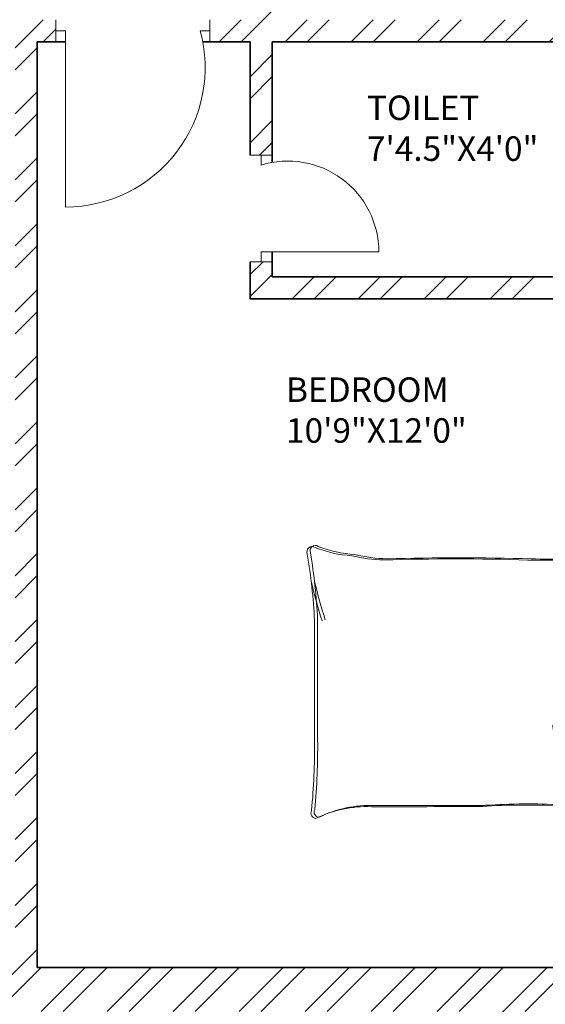
# Model space of a CAD drawing. Units: inches. Extents: x 2120 to 4013, y 1390 to 3019.
# Tile 42 of 59: x 2861 to 2968, y 1964 to 2165. Entities that reach past the tile are written whole.
import ezdxf

# ---------------------------------------------------------------- set-up
doc = ezdxf.new("R2010")
doc.units = ezdxf.units.IN
for name, color, linetype, lineweight in [('A-AREA-IDEN', 7, 'Continuous', 18), ('A-DOOR', 3, 'Continuous', 18), ('A-FURN', 8, 'Continuous', 13), ('A-WALL', 7, 'Continuous', 35), ('A-WALL-PATT', 252, 'Continuous', 13)]:
    doc.layers.add(name, color=color, linetype=linetype, lineweight=lineweight)
doc.styles.get("Standard").update_dxf_attribs({"font": 'arial.ttf'})

# ---------------------------------------------------------------- blocks, each defined once
blk = doc.blocks.new('BED-DOUBLE-PLAN')
for p, q in [((3.48, 63.34), (3.48, 81.45)), ((3.48, 81.45), (51.27, 81.45)), ((3.7, 62.7), (3.7, 80.81)), ((51.27, 81.45), (51.27, 54.84)), ((51.5, 80.81), (51.5, 54.2)), ((3.48, 79.91), (51.27, 79.91)), ((3.7, 79.27), (51.5, 79.27)), ((3.9, 78.11), (8.18, 78.44)), ((8.18, 78.44), (8.29, 78.42)), ((8.29, 78.42), (12.11, 78.13)), ((14.86, 77.7), (16.88, 78.42)), ((16.88, 78.42), (19.77, 79.14)), ((17.11, 77.78), (20, 78.5)), ((19.77, 79.14), (20.09, 79.14)), ((20, 78.5), (20.32, 78.5)), ((20.09, 79.14), (24.54, 79)), ((20.32, 78.5), (24.77, 78.36)), ((24.54, 79), (25.98, 79.58)), ((24.77, 78.36), (26.21, 78.94)), ((25.98, 79.58), (26.56, 74.23)), ((26.21, 78.94), (26.79, 73.59)), ((27.98, 78.95), (27.73, 73.58)), ((29.46, 78.47), (27.98, 78.95)), ((33.89, 78.89), (29.46, 78.47)), ((34.21, 78.91), (33.89, 78.89)), ((37.14, 78.37), (34.21, 78.91)), ((45.71, 78.9), (41.92, 78.38)), ((50.11, 78.89), (44.71, 78.99)), ((44.71, 78.99), (45.71, 78.9)), ((50.11, 78.89), (49.73, 75.68)), ((3.9, 78.13), (4.47, 74.95)), ((4.12, 77.49), (4.7, 74.31)), ((4.13, 77.47), (8.41, 77.8)), ((8.41, 77.8), (8.51, 77.78)), ((8.51, 77.78), (12.34, 77.49)), ((12.11, 78.13), (17.6, 77.12)), ((12.34, 77.49), (17.83, 76.48)), ((15.08, 77.06), (17.11, 77.78)), ((28.21, 78.32), (27.96, 72.94)), ((29.69, 77.83), (28.21, 78.32)), ((34.11, 78.25), (29.69, 77.83)), ((34.43, 78.27), (34.11, 78.25)), ((37.37, 77.73), (34.43, 78.27)), ((41.92, 78.38), (36.5, 77.02)), ((42.14, 77.74), (36.72, 76.38)), ((39.2, 77.77), (37.14, 78.37)), ((39.43, 77.13), (37.37, 77.73)), ((45.94, 78.26), (42.14, 77.74)), ((50.34, 78.25), (44.94, 78.35)), ((44.94, 78.35), (45.94, 78.26)), ((50.34, 78.25), (49.96, 75.04)), ((4.47, 74.95), (4.04, 72.35)), ((5.05, 72.49), (6.06, 75.24)), ((5.28, 71.85), (6.29, 74.6)), ((49.31, 73.19), (48.13, 75.87)), ((49.54, 72.55), (48.36, 75.23)), ((49.73, 75.68), (50.33, 73.11)), ((49.96, 75.04), (50.56, 72.47)), ((4.7, 74.31), (4.27, 71.71)), ((4.47, 68.88), (5.05, 72.49)), ((26.56, 74.23), (27.14, 71.05)), ((26.79, 73.59), (27.37, 70.41)), ((27.73, 73.58), (27.36, 70.37)), ((27.96, 72.94), (27.58, 69.73)), ((50.11, 69.62), (49.31, 73.19)), ((50.34, 68.98), (49.54, 72.55)), ((50.33, 73.11), (49.82, 72.06)), ((50.56, 72.47), (50.04, 71.42)), ((4.04, 72.35), (4.62, 71.33)), ((4.27, 71.71), (4.85, 70.7)), ((4.7, 68.24), (5.28, 71.85)), ((27.14, 71.05), (27.14, 69.74)), ((27.36, 70.37), (27.44, 69.07)), ((27.37, 70.41), (27.37, 69.1)), ((4.76, 67.29), (4.47, 68.88)), ((27.14, 69.74), (26.56, 67.86)), ((27.37, 69.1), (26.79, 67.23)), ((27.44, 69.07), (28.13, 67.23)), ((27.58, 69.73), (27.67, 68.43)), ((27.67, 68.43), (28.36, 66.59)), ((49.92, 68.01), (50.11, 69.62)), ((50.15, 67.37), (50.34, 68.98)), ((4.19, 64.11), (4.76, 67.29)), ((4.41, 63.47), (4.99, 66.65)), ((4.99, 66.65), (4.7, 68.24)), ((26.56, 67.86), (26.56, 65.18)), ((26.79, 67.23), (26.79, 64.54)), ((28.13, 67.23), (28.3, 64.55)), ((28.36, 66.59), (28.53, 63.91)), ((50.7, 64.87), (49.92, 68.01)), ((50.93, 64.23), (50.15, 67.37)), ((9.28, 64.83), (4.19, 64.11)), ((6.38, 65.82), (10.42, 65.15)), ((6.61, 65.18), (10.64, 64.51)), ((10.42, 65.15), (9.28, 64.83)), ((10.64, 64.51), (9.51, 64.19)), ((10.42, 65.15), (17.43, 64.72)), ((10.64, 64.51), (17.65, 64.08)), ((17.43, 64.72), (19.39, 65.28)), ((17.65, 64.08), (19.61, 64.64)), ((19.39, 65.28), (24.52, 64.87)), ((19.61, 64.64), (24.75, 64.23)), ((24.1, 65.18), (20.96, 66.27)), ((24.33, 64.54), (21.19, 65.63)), ((26.56, 65.18), (24.1, 65.18)), ((26.79, 64.54), (24.33, 64.54)), ((28.3, 64.55), (30.75, 64.71)), ((30.75, 64.71), (33.82, 65.99)), ((30.98, 64.07), (34.05, 65.35)), ((32.57, 65.82), (36.6, 65.15)), ((32.79, 65.18), (36.83, 64.51)), ((36.6, 65.15), (43.61, 64.72)), ((36.83, 64.51), (43.84, 64.08)), ((43.61, 64.72), (45.57, 65.28)), ((43.84, 64.08), (45.8, 64.64)), ((45.57, 65.28), (50.7, 64.87)), ((45.8, 64.64), (50.93, 64.23)), ((9.51, 64.19), (4.41, 63.47)), ((28.53, 63.91), (30.98, 64.07)), ((30.26, 64.06), (34.45, 57.57)), ((30.49, 63.42), (34.68, 56.93)), ((40.65, 61.13), (32.31, 64.06)), ((40.87, 60.49), (32.54, 63.42)), ((46.22, 59.12), (40.65, 61.13)), ((46.45, 58.48), (40.87, 60.49)), ((49.16, 56.95), (46.22, 59.12)), ((49.39, 56.31), (46.45, 58.48)), ((34.45, 57.57), (36.15, 53.08)), ((34.68, 56.93), (36.38, 52.44)), ((52.87, 53.7), (49.16, 56.95)), ((53.1, 53.06), (49.39, 56.31)), ((36.15, 53.08), (36.46, 51.07)), ((36.38, 52.44), (36.69, 50.43)), ((38.94, 51.69), (40.96, 52.62)), ((40.96, 52.62), (44.36, 53.08)), ((41.18, 51.98), (44.59, 52.44)), ((44.36, 53.08), (48.23, 53.39)), ((44.59, 52.44), (48.46, 52.75)), ((48.23, 53.39), (51.33, 53.08)), ((48.46, 52.75), (51.56, 52.44)), ((51.33, 53.08), (52.87, 53.7)), ((51.56, 52.44), (53.1, 53.06)), ((52.95, 51.96), (52.87, 53.7, 3.87)), ((53.18, 51.32), (53.1, 53.06, 3.87)), ((36.46, 51.07), (38.94, 51.69)), ((36.69, 50.43), (39.17, 51.05)), ((39.17, 51.05), (41.18, 51.98)), ((15.06, 2.2), (39.68, 2.2)), ((15.29, 1.56), (39.91, 1.56))]:
    blk.add_line(p, q)
for centre, radius, start, end in [((21.36, -100.61), 164.97, 86.0865, 96.7821), ((85.16, 61.35), 83.31, 178.7218, 185.604), ((85.39, 60.71), 83.31, 178.7218, 185.604), ((21.59, -101.25), 164.97, 86.0865, 96.7821), ((17.76, -74.87), 129.02, 81.7845, 96.9006), ((17.99, -75.51), 129.02, 81.7845, 96.9006), ((-167.31, 50.27), 170.11, 358.4762, 1.0082), ((-167.08, 49.63), 170.11, 358.4762, 1.0082), ((43.74, 46.38), 6.22, 78.6608, 113.7384), ((51.33, 88.1), 36.18, 259.8763, 272.5657), ((36.64, 51.01), 0.185, 160.2464, 271.1377), ((31.16, 79.96), 29.65, 280.6617, 289.8806), ((36.87, 50.37), 0.185, 160.2464, 271.1377), ((31.38, 79.32), 29.65, 280.6617, 289.8806), ((43.97, 45.74), 6.22, 78.6608, 113.7384), ((51.56, 87.46), 36.18, 259.8763, 272.5657), ((182.27, 45.13), 129.5, 176.9791, 183.8365), ((182.5, 44.49), 129.5, 176.9791, 183.8365), ((484.82, 30.83), 482.31, 178.2277, 181.7185), ((485.05, 30.19), 482.31, 178.2277, 181.7185), ((-4508.74, 13.62), 4561.86, 0.00217, 0.28689), ((-4508.51, 12.99), 4561.86, 0.00217, 0.28689), ((-26.9, 16.93), 29.63, 346.0648, 358.9113), ((-26.67, 16.29), 29.63, 346.0648, 358.9113), ((76.16, 12.78), 23.07, 177.4714, 206.4681), ((76.39, 12.14), 23.07, 177.4714, 206.4681), ((-21.66, 11.17), 23.56, 337.9751, 356.652), ((-21.43, 10.53), 23.56, 337.9751, 356.652), ((1.09, 1.73), 1.09, 146.1736, 293.4781), ((21.43, -119.39), 121.76, 92.9958, 99.4091), ((-17.22, 105.16), 106.46, 283.3832, 287.7053), ((-16.99, 104.52), 106.46, 283.3832, 287.7053), ((41.15, -130.83), 133.04, 84.4998, 90.6351), ((54.41, 2.58), 1.1, 242.6588, 356.02), ((1.32, 1.09), 1.09, 146.1736, 293.4781), ((21.66, -120.03), 121.76, 92.9958, 99.4091), ((41.38, -131.47), 133.04, 84.4998, 90.6351), ((54.64, 1.94), 1.1, 242.6588, 356.02)]:
    blk.add_arc(centre, radius, start, end)
blk = doc.blocks.new('DOOR-SWING-24IN-107p06DEG')
for p, q in [((0, 21.74), (4.5, 21.74)), ((4.5, 21.74), (2.25, 21.74)), ((2.25, 21.74), (2.25, 19.74)), ((4.5, 0), (0, 0)), ((0, 0), (0, 0)), ((0, 0), (2.25, 0)), ((2.25, 0), (2.25, 2)), ((2.25, 2), (26.25, 2))]:
    blk.add_line(p, q)
blk.add_arc((7.69, 2), 18.56, 0, 107.0611)
blk = doc.blocks.new('DOOR-SWING-36IN-105p32DEG')
for p, q in [((0, 33.75), (0, 38.25)), ((0, 38.25), (0, 36)), ((31.46, 33.75), (31.46, 38.25)), ((31.46, 38.25), (31.46, 36)), ((0, 36), (2, 36)), ((2, 36), (2, 0)), ((31.46, 36), (29.46, 36))]:
    blk.add_line(p, q)
blk.add_arc((2, 28.48), 28.48, 270, 15.3194)

msp = doc.modelspace()

# ---------------------------------------------------------------- hatches: boundary and pattern name
at = {"layer": 'A-WALL-PATT'}
h = msp.add_hatch(dxfattribs=at)
h.set_pattern_fill('ANSI32', color=256)
h.paths.add_polyline_path([(2271.7331, 2343.531), (2283.3788, 2343.531), (2283.3788, 2348.031), (2283.3788, 2352.5306), (2262.7331, 2352.5306), (2262.7331, 2182.638), (2267.2331, 2182.638), (2271.7331, 2182.638), (2271.7331, 2219.031), (2391.7331, 2219.031), (2391.7331, 2214.189), (2393.9831, 2214.189), (2396.2331, 2214.189), (2396.2331, 2219.031), (2420.2331, 2219.031), (2420.2331, 2225.7535), (2417.2197, 2225.7535), (2415.7331, 2225.7535), (2415.7331, 2223.5306), (2271.7331, 2223.5306)])
h.paths.add_polyline_path([(2380.0942, 2352.5306), (2343.3788, 2352.5306), (2343.3788, 2343.531), (2363.2331, 2343.531), (2363.2331, 2288.8489), (2365.4831, 2288.8489), (2367.7331, 2288.8489), (2367.7331, 2343.531), (2380.0942, 2343.531)], flags=17)
h.paths.add_polyline_path([(2432.4339, 2352.5306), (2404.0943, 2352.5306), (2404.0943, 2343.531), (2415.7331, 2343.531), (2415.7331, 2264.0306), (2367.7331, 2264.0306), (2367.7331, 2266.4872), (2363.2331, 2266.4872), (2363.2331, 2259.531), (2367.7331, 2259.531), (2415.7331, 2259.531), (2415.7331, 2255.0658), (2420.2331, 2255.0658), (2420.2331, 2259.531), (2424.5717, 2259.531), (2424.5717, 2261.781), (2424.5717, 2264.0306), (2420.2331, 2264.0306), (2420.2331, 2343.531), (2432.4339, 2343.531)])
h.paths.add_polyline_path([(2508.9115, 2352.5306), (2456.4339, 2352.5306), (2456.4339, 2343.531), (2468.2331, 2343.531), (2468.2331, 2264.0306), (2448.0487, 2264.0306), (2448.0487, 2259.531), (2468.2331, 2259.531), (2468.2331, 2255.5496), (2472.7331, 2255.5496), (2472.7331, 2343.531), (2508.9115, 2343.531)])
h.paths.add_polyline_path([(2637.7331, 2352.5306), (2544.9116, 2352.5306), (2544.9116, 2343.531), (2589.7331, 2343.531), (2633.2331, 2343.531), (2637.7331, 2343.531)])
h.paths.add_polyline_path([(2594.2331, 2343.5306), (2589.7331, 2343.5306), (2589.7331, 2259.5306), (2589.7331, 2252.4915), (2591.9831, 2252.4915), (2594.2331, 2252.4915)])
h.paths.add_polyline_path([(2637.7331, 2223.5306), (2594.2331, 2223.5306), (2594.2331, 2230.1988), (2591.9831, 2230.1988), (2589.7331, 2230.1988), (2589.7331, 2223.5306), (2472.7331, 2223.5306), (2468.2331, 2223.5306), (2468.2331, 2219.031), (2628.7331, 2219.031), (2628.7331, 2138.031), (2637.7331, 2138.031)])
h.paths.add_polyline_path([(3822.6535, 2458.4402), (3874.9468, 2458.4402), (3874.9468, 2476.9866), (3822.6535, 2476.9866)], flags=9)
h.paths.add_polyline_path([(3834.6921, 2781.8174), (3935.9206, 2781.8174), (3935.9206, 2800.3638), (3834.6921, 2800.3638)], flags=9)
h.paths.add_polyline_path([(3832.2843, 2837.9683), (3884.5776, 2837.9683), (3884.5776, 2856.5146), (3832.2843, 2856.5146)], flags=9)
h.paths.add_polyline_path([(3830.9388, 2861.4782), (3956.8958, 2861.4782), (3956.8958, 2880.0245), (3830.9388, 2880.0245)], flags=9)
h.paths.add_polyline_path([(3870.6966, 2352.5752), (3887.9272, 2352.5752), (3887.9272, 2377.3037), (3870.6966, 2377.3037)], flags=9)
h.paths.add_polyline_path([(3289.2701, 2413.161), (3435.2223, 2413.161), (3435.2223, 2450.2538), (3289.2701, 2450.2538)], flags=9)
h.paths.add_polyline_path([(2487.6944, 2414.3601), (2637.8335, 2414.3601), (2637.8335, 2451.4528), (2487.6944, 2451.4528)], flags=9)
h.paths.add_polyline_path([(2567.3724, 1457.9199), (2815.296, 1457.9199), (2815.296, 1495.0127), (2567.3724, 1495.0127)], flags=9)
h.paths.add_polyline_path([(2655.3825, 2093.2363), (2685.9555, 2093.2363), (2685.9555, 2111.8937), (2655.3825, 2111.8937)], flags=9)
h.paths.add_polyline_path([(2543.9218, 1550.6671), (2587.8406, 1550.6671), (2587.8406, 1569.3244), (2543.9218, 1569.3244)], flags=9)
h.paths.add_polyline_path([(2905.1384, 1543.8113), (2949.0572, 1543.8113), (2949.0572, 1562.4686), (2905.1384, 1562.4686)], flags=9)
h.paths.add_polyline_path([(2736.4118, 1702.4736), (2784.2153, 1702.4736), (2784.2153, 1721.1309), (2736.4118, 1721.1309)], flags=9)
h.paths.add_polyline_path([(2912.8666, 1710.4168), (2951.707, 1710.4168), (2951.707, 1729.0741), (2912.8666, 1729.0741)], flags=9)
h.paths.add_polyline_path([(2923.5785, 1763.5038), (2959.7279, 1763.5038), (2959.7279, 1782.1611), (2923.5785, 1782.1611)], flags=9)
h.paths.add_polyline_path([(2925.2114, 1809.6137), (2967.1861, 1809.6137), (2967.1861, 1828.271), (2925.2114, 1828.271)], flags=9)
h.paths.add_polyline_path([(2996.2711, 1878.9003), (2996.2711, 1913.109), (2977.6138, 1913.109), (2977.6138, 1878.9003)], flags=9)
h.paths.add_polyline_path([(2883.0859, 1895.7192), (2927.1855, 1895.7192), (2927.1855, 1914.3766), (2883.0859, 1914.3766)], flags=9)
h.paths.add_polyline_path([(2787.3924, 1810.8013), (2841.0213, 1810.8013), (2841.0213, 1829.4587), (2787.3924, 1829.4587)], flags=9)
h.paths.add_polyline_path([(2775.6399, 2101.7395), (2829.2689, 2101.7395), (2829.2689, 2120.3968), (2775.6399, 2120.3968)], flags=9)
h.paths.add_polyline_path([(2913.0263, 2075.817), (2951.8667, 2075.817), (2951.8667, 2094.4744), (2913.0263, 2094.4744)], flags=9)
h.paths.add_polyline_path([(2929.966, 2133.3669), (2966.1154, 2133.3669), (2966.1154, 2152.0243), (2929.966, 2152.0243)], flags=9)
h.paths.add_polyline_path([(2932.7502, 2182.6088), (2968.8996, 2182.6088), (2968.8996, 2201.2662), (2932.7502, 2201.2662)], flags=9)
h.paths.add_polyline_path([(2996.0681, 2266.3173), (2996.0681, 2300.5261), (2977.4108, 2300.5261), (2977.4108, 2266.3173)], flags=9)
h.paths.add_polyline_path([(2885.1039, 2279.2186), (2929.2035, 2279.2186), (2929.2035, 2297.8759), (2885.1039, 2297.8759)], flags=9)
h.paths.add_polyline_path([(2735.7042, 2218.3197), (2783.5078, 2218.3197), (2783.5078, 2236.9771), (2735.7042, 2236.9771)], flags=9)
h.paths.add_polyline_path([(2635.6049, 2044.0085), (2648.9678, 2044.0085), (2648.9678, 2054.312), (2635.6049, 2054.312)], flags=9)
h.paths.add_polyline_path([(2714.0148, 1923.0473), (2727.3777, 1923.0473), (2727.3777, 1933.3508), (2714.0148, 1933.3508)], flags=9)
h.paths.add_polyline_path([(2709.0345, 1988.1628), (2722.3974, 1988.1628), (2722.3974, 1998.4663), (2709.0345, 1998.4663)], flags=9)
h.paths.add_polyline_path([(2592.8935, 1962.1763), (2606.2564, 1962.1763), (2606.2564, 1972.4799), (2592.8935, 1972.4799)], flags=9)
h.paths.add_polyline_path([(2618.3996, 1985.9724), (2644.1942, 1985.9724), (2644.1942, 1996.2759), (2618.3996, 1996.2759)], flags=9)
h.paths.add_polyline_path([(2601.279, 1920.5869), (2614.6419, 1920.5869), (2614.6419, 1930.8904), (2601.279, 1930.8904)], flags=9)
h.paths.add_polyline_path([(2692.3278, 1932.7645), (2704.5311, 1932.7645), (2704.5311, 1943.0681), (2692.3278, 1943.0681)], flags=9)
h.paths.add_polyline_path([(2311.122, 1672.7318), (2355.0408, 1672.7318), (2355.0408, 1691.3892), (2311.122, 1691.3892)], flags=9)
h.paths.add_polyline_path([(2456.2551, 1632.3198), (2492.4796, 1632.3198), (2492.4796, 1650.9772), (2456.2551, 1650.9772)], flags=9)
h.paths.add_polyline_path([(2401.0766, 1631.4793), (2437.301, 1631.4793), (2437.301, 1650.1367), (2401.0766, 1650.1367)], flags=9)
h.paths.add_polyline_path([(2546.7054, 1700.9235), (2594.509, 1700.9235), (2594.509, 1719.5809), (2546.7054, 1719.5809)], flags=9)
h.paths.add_polyline_path([(2445.4866, 1766.9937), (2497.5261, 1766.9937), (2497.5261, 1785.651), (2445.4866, 1785.651)], flags=9)
h.paths.add_polyline_path([(2287.9992, 1739.7675), (2326.8396, 1739.7675), (2326.8396, 1758.4248), (2287.9992, 1758.4248)], flags=9)
h.paths.add_polyline_path([(2458.5279, 1924.7607), (2510.5675, 1924.7607), (2510.5675, 1943.4181), (2458.5279, 1943.4181)], flags=9)
h.paths.add_polyline_path([(2309.2811, 1902.7642), (2345.4305, 1902.7642), (2345.4305, 1921.4215), (2309.2811, 1921.4215)], flags=9)
h.paths.add_polyline_path([(2490.7554, 2018.9392), (2530.7896, 2018.9392), (2530.7896, 2037.5965), (2490.7554, 2037.5965)], flags=9)
h.paths.add_polyline_path([(2402.143, 2024.7393), (2438.5414, 2024.7393), (2438.5414, 2043.3966), (2402.143, 2043.3966)], flags=9)
h.paths.add_polyline_path([(2287.856, 1931.7926), (2326.6964, 1931.7926), (2326.6964, 1950.4499), (2287.856, 1950.4499)], flags=9)
h.paths.add_polyline_path([(2281.7979, 2193.5771), (2320.6383, 2193.5771), (2320.6383, 2212.2344), (2281.7979, 2212.2344)], flags=25)
h.paths.add_polyline_path([(2484.0754, 2093.892), (2536.115, 2093.892), (2536.115, 2112.5494), (2484.0754, 2112.5494)], flags=9)
h.paths.add_polyline_path([(2624.7948, 2281.8639), (2624.7948, 2311.4137), (2606.1375, 2311.4137), (2606.1375, 2281.8639)], flags=9)
h.paths.add_polyline_path([(2507.5036, 2290.3639), (2541.934, 2290.3639), (2541.934, 2309.0212), (2507.5036, 2309.0212)], flags=9)
h.paths.add_polyline_path([(2423.1076, 2285.2202), (2459.332, 2285.2202), (2459.332, 2303.8776), (2423.1076, 2303.8776)], flags=9)
h.paths.add_polyline_path([(2374.5467, 2289.6272), (2410.7711, 2289.6272), (2410.7711, 2308.2846), (2374.5467, 2308.2846)], flags=25)
h.paths.add_polyline_path([(2277.4907, 2227.5651), (2316.3311, 2227.5651), (2316.3311, 2246.2224), (2277.4907, 2246.2224)], flags=25)
h.paths.add_polyline_path([(2655.3825, 2093.2367), (2685.9555, 2093.2367), (2685.9555, 2111.894), (2655.3825, 2111.894)], flags=9)
h.paths.add_polyline_path([(2543.9217, 1550.6674), (2587.8406, 1550.6674), (2587.8406, 1569.3247), (2543.9217, 1569.3247)], flags=9)
h.paths.add_polyline_path([(2905.1384, 1543.8116), (2949.0572, 1543.8116), (2949.0572, 1562.4689), (2905.1384, 1562.4689)], flags=9)
h.paths.add_polyline_path([(2736.4118, 1702.4739), (2784.2153, 1702.4739), (2784.2153, 1721.1312), (2736.4118, 1721.1312)], flags=9)
h.paths.add_polyline_path([(2912.8666, 1710.4171), (2951.707, 1710.4171), (2951.707, 1729.0744), (2912.8666, 1729.0744)], flags=9)
h.paths.add_polyline_path([(2923.5785, 1763.5041), (2959.7279, 1763.5041), (2959.7279, 1782.1614), (2923.5785, 1782.1614)], flags=9)
h.paths.add_polyline_path([(2925.2114, 1809.614), (2967.1861, 1809.614), (2967.1861, 1828.2713), (2925.2114, 1828.2713)], flags=9)
h.paths.add_polyline_path([(2996.2711, 1878.9006), (2996.2711, 1913.1094), (2977.6137, 1913.1094), (2977.6137, 1878.9006)], flags=9)
h.paths.add_polyline_path([(2883.0859, 1895.7195), (2927.1855, 1895.7195), (2927.1855, 1914.3769), (2883.0859, 1914.3769)], flags=9)
h.paths.add_polyline_path([(2787.3924, 1810.8016), (2841.0213, 1810.8016), (2841.0213, 1829.459), (2787.3924, 1829.459)], flags=9)
h.paths.add_polyline_path([(2775.6399, 2101.7398), (2829.2688, 2101.7398), (2829.2688, 2120.3971), (2775.6399, 2120.3971)], flags=9)
h.paths.add_polyline_path([(2913.0263, 2075.8173), (2951.8667, 2075.8173), (2951.8667, 2094.4747), (2913.0263, 2094.4747)], flags=9)
h.paths.add_polyline_path([(2929.966, 2133.3672), (2966.1154, 2133.3672), (2966.1154, 2152.0246), (2929.966, 2152.0246)], flags=9)
h.paths.add_polyline_path([(2932.7502, 2182.6091), (2968.8996, 2182.6091), (2968.8996, 2201.2665), (2932.7502, 2201.2665)], flags=9)
h.paths.add_polyline_path([(2996.0681, 2266.3176), (2996.0681, 2300.5264), (2977.4108, 2300.5264), (2977.4108, 2266.3176)], flags=9)
h.paths.add_polyline_path([(2885.1039, 2279.2189), (2929.2035, 2279.2189), (2929.2035, 2297.8762), (2885.1039, 2297.8762)], flags=9)
h.paths.add_polyline_path([(2735.7042, 2218.32), (2783.5078, 2218.32), (2783.5078, 2236.9774), (2735.7042, 2236.9774)], flags=9)
h.paths.add_polyline_path([(2635.6048, 2044.0088), (2648.9677, 2044.0088), (2648.9677, 2054.3123), (2635.6048, 2054.3123)], flags=9)
h.paths.add_polyline_path([(2714.0148, 1923.0476), (2727.3777, 1923.0476), (2727.3777, 1933.3511), (2714.0148, 1933.3511)], flags=9)
h.paths.add_polyline_path([(2709.0345, 1988.1631), (2722.3974, 1988.1631), (2722.3974, 1998.4666), (2709.0345, 1998.4666)], flags=9)
h.paths.add_polyline_path([(2592.8935, 1962.1766), (2606.2564, 1962.1766), (2606.2564, 1972.4802), (2592.8935, 1972.4802)], flags=9)
h.paths.add_polyline_path([(2618.3995, 1985.9727), (2644.1942, 1985.9727), (2644.1942, 1996.2762), (2618.3995, 1996.2762)], flags=9)
h.paths.add_polyline_path([(2601.279, 1920.5872), (2614.6419, 1920.5872), (2614.6419, 1930.8908), (2601.279, 1930.8908)], flags=9)
h.paths.add_polyline_path([(2692.3278, 1932.7648), (2704.5311, 1932.7648), (2704.5311, 1943.0684), (2692.3278, 1943.0684)], flags=9)
h.paths.add_polyline_path([(2311.122, 1672.7321), (2355.0408, 1672.7321), (2355.0408, 1691.3895), (2311.122, 1691.3895)], flags=9)
h.paths.add_polyline_path([(2456.2551, 1632.3201), (2492.4795, 1632.3201), (2492.4795, 1650.9775), (2456.2551, 1650.9775)], flags=9)
h.paths.add_polyline_path([(2401.0766, 1631.4796), (2437.301, 1631.4796), (2437.301, 1650.137), (2401.0766, 1650.137)], flags=9)
h.paths.add_polyline_path([(2546.7054, 1700.9238), (2594.509, 1700.9238), (2594.509, 1719.5812), (2546.7054, 1719.5812)], flags=9)
h.paths.add_polyline_path([(2445.4866, 1766.994), (2497.5261, 1766.994), (2497.5261, 1785.6513), (2445.4866, 1785.6513)], flags=9)
h.paths.add_polyline_path([(2287.9992, 1739.7678), (2326.8396, 1739.7678), (2326.8396, 1758.4251), (2287.9992, 1758.4251)], flags=9)
h.paths.add_polyline_path([(2458.5279, 1924.7611), (2510.5675, 1924.7611), (2510.5675, 1943.4184), (2458.5279, 1943.4184)], flags=9)
h.paths.add_polyline_path([(2309.2811, 1902.7645), (2345.4305, 1902.7645), (2345.4305, 1921.4218), (2309.2811, 1921.4218)], flags=9)
h.paths.add_polyline_path([(2490.7554, 2018.9395), (2530.7895, 2018.9395), (2530.7895, 2037.5968), (2490.7554, 2037.5968)], flags=9)
h.paths.add_polyline_path([(2402.143, 2024.7396), (2438.5413, 2024.7396), (2438.5413, 2043.3969), (2402.143, 2043.3969)], flags=9)
h.paths.add_polyline_path([(2287.856, 1931.7929), (2326.6964, 1931.7929), (2326.6964, 1950.4502), (2287.856, 1950.4502)], flags=9)
h.paths.add_polyline_path([(2281.7979, 2193.5774), (2320.6383, 2193.5774), (2320.6383, 2212.2347), (2281.7979, 2212.2347)], flags=25)
h.paths.add_polyline_path([(2484.0754, 2093.8924), (2536.115, 2093.8924), (2536.115, 2112.5497), (2484.0754, 2112.5497)], flags=9)
h.paths.add_polyline_path([(2624.7948, 2281.8642), (2624.7948, 2311.414), (2606.1374, 2311.414), (2606.1374, 2281.8642)], flags=9)
h.paths.add_polyline_path([(2507.5035, 2290.3642), (2541.934, 2290.3642), (2541.934, 2309.0215), (2507.5035, 2309.0215)], flags=9)
h.paths.add_polyline_path([(2423.1075, 2285.2205), (2459.332, 2285.2205), (2459.332, 2303.8779), (2423.1075, 2303.8779)], flags=9)
h.paths.add_polyline_path([(2374.5467, 2289.6275), (2410.7711, 2289.6275), (2410.7711, 2308.2849), (2374.5467, 2308.2849)], flags=25)
h.paths.add_polyline_path([(2277.4907, 2227.5654), (2316.3311, 2227.5654), (2316.3311, 2246.2227), (2277.4907, 2246.2227)], flags=25)
h = msp.add_hatch(dxfattribs=at)
h.set_pattern_fill('ANSI32', color=256)
h.paths.add_polyline_path([(2271.7331, 1980.389), (2262.7331, 1980.389), (2262.7331, 1912.8434), (2267.2331, 1912.8434), (2271.7331, 1912.8434), (2271.7331, 1922.531), (2351.2331, 1922.531), (2351.2331, 1901.4728), (2355.7331, 1901.4728), (2355.7331, 1922.531), (2357.9815, 1922.531), (2357.9815, 1926.5306), (2271.7331, 1926.5306)])
h.paths.add_polyline_path([(2589.2331, 1949.1622), (2584.7331, 1949.1622), (2580.2331, 1949.1622), (2580.2331, 1874.5306), (2355.7331, 1874.5306), (2355.7331, 1880.1922), (2351.2331, 1880.1922), (2351.2331, 1874.5306), (2271.7331, 1874.5306), (2271.7331, 1888.8431), (2262.7331, 1888.8431), (2262.7331, 1842.2909), (2267.2331, 1842.2909), (2271.7331, 1842.2909), (2271.7331, 1865.531), (2415.7331, 1865.531), (2415.7331, 1779.7286), (2420.2331, 1779.7286), (2420.2331, 1865.531), (2589.2331, 1865.531)])
h.paths.add_polyline_path([(2271.7331, 1782.2906), (2262.7331, 1782.2906), (2262.7331, 1711.4639), (2267.2331, 1711.4639), (2271.7331, 1711.4639), (2271.7331, 1738.031), (2420.2331, 1738.031), (2420.2331, 1742.531), (2420.2331, 1747.3376), (2417.9831, 1747.3376), (2415.7331, 1747.3376), (2415.7331, 1742.5306), (2271.7331, 1742.5306)])
h.paths.add_polyline_path([(2271.7331, 1627.031), (2362.3957, 1627.031), (2362.3957, 1629.281), (2362.3957, 1631.5306), (2271.7331, 1631.5306), (2271.7331, 1675.4636), (2262.7331, 1675.4636), (2262.7331, 1581.531), (2405.3032, 1581.531), (2405.3032, 1586.031), (2405.3032, 1590.5306), (2396.2331, 1590.5306), (2396.2331, 1691.4513), (2418.7206, 1691.4513), (2418.7206, 1695.951), (2396.2331, 1695.951), (2391.7331, 1695.951), (2391.7331, 1631.5306), (2386.7425, 1631.5306), (2386.7425, 1629.2806), (2386.7425, 1627.031), (2391.7331, 1627.031), (2391.7331, 1586.1709), (2271.7331, 1586.1709)])
h.paths.add_polyline_path([(2459.6703, 1590.5306), (2429.3032, 1590.5306), (2429.3032, 1581.531), (2459.6703, 1581.531), (2459.6703, 1586.031)])
h.paths.add_polyline_path([(2501.2331, 1590.531), (2501.2331, 1665.0195), (2498.9831, 1665.0195), (2496.7331, 1665.0195), (2496.7331, 1590.5306), (2483.8201, 1590.5306), (2483.8201, 1590.1579), (2483.6704, 1590.1579), (2483.6704, 1581.531), (2505.0196, 1581.531), (2505.0196, 1583.781), (2505.0196, 1586.0306), (2501.2331, 1586.0306)])
h.paths.add_polyline_path([(2544.1361, 1583.781), (2544.1361, 1586.0306), (2527.1368, 1586.0306), (2527.1368, 1583.7806), (2527.1368, 1581.531), (2544.1361, 1581.531)])
h.paths.add_polyline_path([(3822.6535, 2458.4402), (3874.9468, 2458.4402), (3874.9468, 2476.9866), (3822.6535, 2476.9866)], flags=9)
h.paths.add_polyline_path([(3834.6921, 2781.8174), (3935.9206, 2781.8174), (3935.9206, 2800.3638), (3834.6921, 2800.3638)], flags=9)
h.paths.add_polyline_path([(3832.2843, 2837.9683), (3884.5776, 2837.9683), (3884.5776, 2856.5146), (3832.2843, 2856.5146)], flags=9)
h.paths.add_polyline_path([(3830.9388, 2861.4782), (3956.8958, 2861.4782), (3956.8958, 2880.0245), (3830.9388, 2880.0245)], flags=9)
h.paths.add_polyline_path([(3870.6966, 2352.5752), (3887.9272, 2352.5752), (3887.9272, 2377.3037), (3870.6966, 2377.3037)], flags=9)
h.paths.add_polyline_path([(3289.2701, 2413.161), (3435.2223, 2413.161), (3435.2223, 2450.2538), (3289.2701, 2450.2538)], flags=9)
h.paths.add_polyline_path([(2487.6944, 2414.3601), (2637.8335, 2414.3601), (2637.8335, 2451.4528), (2487.6944, 2451.4528)], flags=9)
h.paths.add_polyline_path([(2567.3724, 1457.9199), (2815.296, 1457.9199), (2815.296, 1495.0127), (2567.3724, 1495.0127)], flags=9)
h.paths.add_polyline_path([(2655.3825, 2093.2363), (2685.9555, 2093.2363), (2685.9555, 2111.8937), (2655.3825, 2111.8937)], flags=9)
h.paths.add_polyline_path([(2543.9218, 1550.6671), (2587.8406, 1550.6671), (2587.8406, 1569.3244), (2543.9218, 1569.3244)], flags=9)
h.paths.add_polyline_path([(2905.1384, 1543.8113), (2949.0572, 1543.8113), (2949.0572, 1562.4686), (2905.1384, 1562.4686)], flags=9)
h.paths.add_polyline_path([(2736.4118, 1702.4736), (2784.2153, 1702.4736), (2784.2153, 1721.1309), (2736.4118, 1721.1309)], flags=9)
h.paths.add_polyline_path([(2912.8666, 1710.4168), (2951.707, 1710.4168), (2951.707, 1729.0741), (2912.8666, 1729.0741)], flags=9)
h.paths.add_polyline_path([(2923.5785, 1763.5038), (2959.7279, 1763.5038), (2959.7279, 1782.1611), (2923.5785, 1782.1611)], flags=9)
h.paths.add_polyline_path([(2925.2114, 1809.6137), (2967.1861, 1809.6137), (2967.1861, 1828.271), (2925.2114, 1828.271)], flags=9)
h.paths.add_polyline_path([(2996.2711, 1878.9003), (2996.2711, 1913.109), (2977.6138, 1913.109), (2977.6138, 1878.9003)], flags=9)
h.paths.add_polyline_path([(2883.0859, 1895.7192), (2927.1855, 1895.7192), (2927.1855, 1914.3766), (2883.0859, 1914.3766)], flags=9)
h.paths.add_polyline_path([(2787.3924, 1810.8013), (2841.0213, 1810.8013), (2841.0213, 1829.4587), (2787.3924, 1829.4587)], flags=9)
h.paths.add_polyline_path([(2775.6399, 2101.7395), (2829.2689, 2101.7395), (2829.2689, 2120.3968), (2775.6399, 2120.3968)], flags=9)
h.paths.add_polyline_path([(2913.0263, 2075.817), (2951.8667, 2075.817), (2951.8667, 2094.4744), (2913.0263, 2094.4744)], flags=9)
h.paths.add_polyline_path([(2929.966, 2133.3669), (2966.1154, 2133.3669), (2966.1154, 2152.0243), (2929.966, 2152.0243)], flags=9)
h.paths.add_polyline_path([(2932.7502, 2182.6088), (2968.8996, 2182.6088), (2968.8996, 2201.2662), (2932.7502, 2201.2662)], flags=9)
h.paths.add_polyline_path([(2996.0681, 2266.3173), (2996.0681, 2300.5261), (2977.4108, 2300.5261), (2977.4108, 2266.3173)], flags=9)
h.paths.add_polyline_path([(2885.1039, 2279.2186), (2929.2035, 2279.2186), (2929.2035, 2297.8759), (2885.1039, 2297.8759)], flags=9)
h.paths.add_polyline_path([(2735.7042, 2218.3197), (2783.5078, 2218.3197), (2783.5078, 2236.9771), (2735.7042, 2236.9771)], flags=9)
h.paths.add_polyline_path([(2635.6049, 2044.0085), (2648.9678, 2044.0085), (2648.9678, 2054.312), (2635.6049, 2054.312)], flags=9)
h.paths.add_polyline_path([(2714.0148, 1923.0473), (2727.3777, 1923.0473), (2727.3777, 1933.3508), (2714.0148, 1933.3508)], flags=9)
h.paths.add_polyline_path([(2709.0345, 1988.1628), (2722.3974, 1988.1628), (2722.3974, 1998.4663), (2709.0345, 1998.4663)], flags=9)
h.paths.add_polyline_path([(2592.8935, 1962.1763), (2606.2564, 1962.1763), (2606.2564, 1972.4799), (2592.8935, 1972.4799)], flags=9)
h.paths.add_polyline_path([(2618.3996, 1985.9724), (2644.1942, 1985.9724), (2644.1942, 1996.2759), (2618.3996, 1996.2759)], flags=9)
h.paths.add_polyline_path([(2601.279, 1920.5869), (2614.6419, 1920.5869), (2614.6419, 1930.8904), (2601.279, 1930.8904)], flags=9)
h.paths.add_polyline_path([(2692.3278, 1932.7645), (2704.5311, 1932.7645), (2704.5311, 1943.0681), (2692.3278, 1943.0681)], flags=9)
h.paths.add_polyline_path([(2311.122, 1672.7318), (2355.0408, 1672.7318), (2355.0408, 1691.3892), (2311.122, 1691.3892)], flags=25)
h.paths.add_polyline_path([(2456.2551, 1632.3198), (2492.4796, 1632.3198), (2492.4796, 1650.9772), (2456.2551, 1650.9772)], flags=9)
h.paths.add_polyline_path([(2401.0766, 1631.4793), (2437.301, 1631.4793), (2437.301, 1650.1367), (2401.0766, 1650.1367)], flags=9)
h.paths.add_polyline_path([(2546.7054, 1700.9235), (2594.509, 1700.9235), (2594.509, 1719.5809), (2546.7054, 1719.5809)], flags=9)
h.paths.add_polyline_path([(2445.4866, 1766.9937), (2497.5261, 1766.9937), (2497.5261, 1785.651), (2445.4866, 1785.651)], flags=9)
h.paths.add_polyline_path([(2287.9992, 1739.7675), (2326.8396, 1739.7675), (2326.8396, 1758.4248), (2287.9992, 1758.4248)], flags=24)
h.paths.add_polyline_path([(2458.5279, 1924.7607), (2510.5675, 1924.7607), (2510.5675, 1943.4181), (2458.5279, 1943.4181)], flags=25)
h.paths.add_polyline_path([(2309.2811, 1902.7642), (2345.4305, 1902.7642), (2345.4305, 1921.4215), (2309.2811, 1921.4215)], flags=25)
h.paths.add_polyline_path([(2490.7554, 2018.9392), (2530.7896, 2018.9392), (2530.7896, 2037.5965), (2490.7554, 2037.5965)], flags=9)
h.paths.add_polyline_path([(2402.143, 2024.7393), (2438.5414, 2024.7393), (2438.5414, 2043.3966), (2402.143, 2043.3966)], flags=9)
h.paths.add_polyline_path([(2287.856, 1931.7926), (2326.6964, 1931.7926), (2326.6964, 1950.4499), (2287.856, 1950.4499)], flags=25)
h.paths.add_polyline_path([(2281.7979, 2193.5771), (2320.6383, 2193.5771), (2320.6383, 2212.2344), (2281.7979, 2212.2344)], flags=9)
h.paths.add_polyline_path([(2484.0754, 2093.892), (2536.115, 2093.892), (2536.115, 2112.5494), (2484.0754, 2112.5494)], flags=9)
h.paths.add_polyline_path([(2624.7948, 2281.8639), (2624.7948, 2311.4137), (2606.1375, 2311.4137), (2606.1375, 2281.8639)], flags=9)
h.paths.add_polyline_path([(2507.5036, 2290.3639), (2541.934, 2290.3639), (2541.934, 2309.0212), (2507.5036, 2309.0212)], flags=9)
h.paths.add_polyline_path([(2423.1076, 2285.2202), (2459.332, 2285.2202), (2459.332, 2303.8776), (2423.1076, 2303.8776)], flags=9)
h.paths.add_polyline_path([(2374.5467, 2289.6272), (2410.7711, 2289.6272), (2410.7711, 2308.2846), (2374.5467, 2308.2846)], flags=9)
h.paths.add_polyline_path([(2277.4907, 2227.5651), (2316.3311, 2227.5651), (2316.3311, 2246.2224), (2277.4907, 2246.2224)], flags=9)
h.paths.add_polyline_path([(2655.3825, 2093.2367), (2685.9555, 2093.2367), (2685.9555, 2111.894), (2655.3825, 2111.894)], flags=9)
h.paths.add_polyline_path([(2543.9217, 1550.6674), (2587.8406, 1550.6674), (2587.8406, 1569.3247), (2543.9217, 1569.3247)], flags=9)
h.paths.add_polyline_path([(2905.1384, 1543.8116), (2949.0572, 1543.8116), (2949.0572, 1562.4689), (2905.1384, 1562.4689)], flags=9)
h.paths.add_polyline_path([(2736.4118, 1702.4739), (2784.2153, 1702.4739), (2784.2153, 1721.1312), (2736.4118, 1721.1312)], flags=9)
h.paths.add_polyline_path([(2912.8666, 1710.4171), (2951.707, 1710.4171), (2951.707, 1729.0744), (2912.8666, 1729.0744)], flags=9)
h.paths.add_polyline_path([(2923.5785, 1763.5041), (2959.7279, 1763.5041), (2959.7279, 1782.1614), (2923.5785, 1782.1614)], flags=9)
h.paths.add_polyline_path([(2925.2114, 1809.614), (2967.1861, 1809.614), (2967.1861, 1828.2713), (2925.2114, 1828.2713)], flags=9)
h.paths.add_polyline_path([(2996.2711, 1878.9006), (2996.2711, 1913.1094), (2977.6137, 1913.1094), (2977.6137, 1878.9006)], flags=9)
h.paths.add_polyline_path([(2883.0859, 1895.7195), (2927.1855, 1895.7195), (2927.1855, 1914.3769), (2883.0859, 1914.3769)], flags=9)
h.paths.add_polyline_path([(2787.3924, 1810.8016), (2841.0213, 1810.8016), (2841.0213, 1829.459), (2787.3924, 1829.459)], flags=9)
h.paths.add_polyline_path([(2775.6399, 2101.7398), (2829.2688, 2101.7398), (2829.2688, 2120.3971), (2775.6399, 2120.3971)], flags=9)
h.paths.add_polyline_path([(2913.0263, 2075.8173), (2951.8667, 2075.8173), (2951.8667, 2094.4747), (2913.0263, 2094.4747)], flags=9)
h.paths.add_polyline_path([(2929.966, 2133.3672), (2966.1154, 2133.3672), (2966.1154, 2152.0246), (2929.966, 2152.0246)], flags=9)
h.paths.add_polyline_path([(2932.7502, 2182.6091), (2968.8996, 2182.6091), (2968.8996, 2201.2665), (2932.7502, 2201.2665)], flags=9)
h.paths.add_polyline_path([(2996.0681, 2266.3176), (2996.0681, 2300.5264), (2977.4108, 2300.5264), (2977.4108, 2266.3176)], flags=9)
h.paths.add_polyline_path([(2885.1039, 2279.2189), (2929.2035, 2279.2189), (2929.2035, 2297.8762), (2885.1039, 2297.8762)], flags=9)
h.paths.add_polyline_path([(2735.7042, 2218.32), (2783.5078, 2218.32), (2783.5078, 2236.9774), (2735.7042, 2236.9774)], flags=9)
h.paths.add_polyline_path([(2635.6048, 2044.0088), (2648.9677, 2044.0088), (2648.9677, 2054.3123), (2635.6048, 2054.3123)], flags=9)
h.paths.add_polyline_path([(2714.0148, 1923.0476), (2727.3777, 1923.0476), (2727.3777, 1933.3511), (2714.0148, 1933.3511)], flags=9)
h.paths.add_polyline_path([(2709.0345, 1988.1631), (2722.3974, 1988.1631), (2722.3974, 1998.4666), (2709.0345, 1998.4666)], flags=9)
h.paths.add_polyline_path([(2592.8935, 1962.1766), (2606.2564, 1962.1766), (2606.2564, 1972.4802), (2592.8935, 1972.4802)], flags=9)
h.paths.add_polyline_path([(2618.3995, 1985.9727), (2644.1942, 1985.9727), (2644.1942, 1996.2762), (2618.3995, 1996.2762)], flags=9)
h.paths.add_polyline_path([(2601.279, 1920.5872), (2614.6419, 1920.5872), (2614.6419, 1930.8908), (2601.279, 1930.8908)], flags=9)
h.paths.add_polyline_path([(2692.3278, 1932.7648), (2704.5311, 1932.7648), (2704.5311, 1943.0684), (2692.3278, 1943.0684)], flags=9)
h.paths.add_polyline_path([(2311.122, 1672.7321), (2355.0408, 1672.7321), (2355.0408, 1691.3895), (2311.122, 1691.3895)], flags=25)
h.paths.add_polyline_path([(2456.2551, 1632.3201), (2492.4795, 1632.3201), (2492.4795, 1650.9775), (2456.2551, 1650.9775)], flags=9)
h.paths.add_polyline_path([(2401.0766, 1631.4796), (2437.301, 1631.4796), (2437.301, 1650.137), (2401.0766, 1650.137)], flags=9)
h.paths.add_polyline_path([(2546.7054, 1700.9238), (2594.509, 1700.9238), (2594.509, 1719.5812), (2546.7054, 1719.5812)], flags=9)
h.paths.add_polyline_path([(2445.4866, 1766.994), (2497.5261, 1766.994), (2497.5261, 1785.6513), (2445.4866, 1785.6513)], flags=9)
h.paths.add_polyline_path([(2287.9992, 1739.7678), (2326.8396, 1739.7678), (2326.8396, 1758.4251), (2287.9992, 1758.4251)], flags=24)
h.paths.add_polyline_path([(2458.5279, 1924.7611), (2510.5675, 1924.7611), (2510.5675, 1943.4184), (2458.5279, 1943.4184)], flags=25)
h.paths.add_polyline_path([(2309.2811, 1902.7645), (2345.4305, 1902.7645), (2345.4305, 1921.4218), (2309.2811, 1921.4218)], flags=25)
h.paths.add_polyline_path([(2490.7554, 2018.9395), (2530.7895, 2018.9395), (2530.7895, 2037.5968), (2490.7554, 2037.5968)], flags=9)
h.paths.add_polyline_path([(2402.143, 2024.7396), (2438.5413, 2024.7396), (2438.5413, 2043.3969), (2402.143, 2043.3969)], flags=9)
h.paths.add_polyline_path([(2287.856, 1931.7929), (2326.6964, 1931.7929), (2326.6964, 1950.4502), (2287.856, 1950.4502)], flags=25)
h.paths.add_polyline_path([(2281.7979, 2193.5774), (2320.6383, 2193.5774), (2320.6383, 2212.2347), (2281.7979, 2212.2347)], flags=9)
h.paths.add_polyline_path([(2484.0754, 2093.8924), (2536.115, 2093.8924), (2536.115, 2112.5497), (2484.0754, 2112.5497)], flags=9)
h.paths.add_polyline_path([(2624.7948, 2281.8642), (2624.7948, 2311.414), (2606.1374, 2311.414), (2606.1374, 2281.8642)], flags=9)
h.paths.add_polyline_path([(2507.5035, 2290.3642), (2541.934, 2290.3642), (2541.934, 2309.0215), (2507.5035, 2309.0215)], flags=9)
h.paths.add_polyline_path([(2423.1075, 2285.2205), (2459.332, 2285.2205), (2459.332, 2303.8779), (2423.1075, 2303.8779)], flags=9)
h.paths.add_polyline_path([(2374.5467, 2289.6275), (2410.7711, 2289.6275), (2410.7711, 2308.2849), (2374.5467, 2308.2849)], flags=9)
h.paths.add_polyline_path([(2277.4907, 2227.5654), (2316.3311, 2227.5654), (2316.3311, 2246.2227), (2277.4907, 2246.2227)], flags=9)
h = msp.add_hatch(dxfattribs=at)
h.set_pattern_fill('ANSI32', color=256)
h.paths.add_polyline_path([(2271.7331, 2122.6377), (2262.7331, 2122.6377), (2262.7331, 2040.3893), (2267.2331, 2040.3893), (2271.7331, 2040.3893), (2271.7331, 2044.8856), (2271.7331, 2070.531), (2391.7331, 2070.531), (2391.7331, 1926.5306), (2388.3993, 1926.5306), (2388.3993, 1922.531), (2395.7331, 1922.531), (2395.7331, 1992.531), (2400.4511, 1992.531), (2400.4511, 1997.0306), (2395.7331, 1997.0306), (2395.7331, 2070.531), (2443.7331, 2070.531), (2443.7331, 2046.1368), (2448.2331, 2046.1368), (2448.2331, 2070.531), (2580.2331, 2070.531), (2580.2331, 1997.0306), (2492.9076, 1997.0306), (2492.9076, 1992.531), (2580.2331, 1992.531), (2580.2331, 1983.9368), (2589.2331, 1983.9368), (2589.2331, 2070.531), (2589.2331, 2075.0306), (2396.2331, 2075.0306), (2396.2331, 2184.3565), (2393.9831, 2184.3565), (2391.7331, 2184.3565), (2391.7331, 2075.0306), (2271.7331, 2075.0306)])
h.paths.add_polyline_path([(2724.7331, 2138.0306), (2628.7331, 2138.0306), (2628.7331, 2070.5306), (2628.7331, 2067.0987), (2633.2331, 2067.0987), (2637.7331, 2067.0987), (2637.7331, 2070.531), (2657.3413, 2070.531), (2657.3413, 2079.5306), (2637.7331, 2079.5306), (2637.7331, 2129.031), (2715.7331, 2129.031), (2715.7331, 2079.5306), (2698.0378, 2079.5306), (2698.0378, 2070.531), (2715.7331, 2070.531), (2715.7331, 2012.1531), (2720.2331, 2012.1531), (2724.7331, 2012.1531)])
h.paths.add_polyline_path([(2724.7331, 2213.031), (2831.3209, 2213.031), (2831.3209, 2215.281), (2831.3209, 2217.5306), (2724.7331, 2217.5306), (2724.7331, 2343.531), (2751.8755, 2343.531), (2751.8755, 2352.5306), (2715.7331, 2352.5306), (2715.7331, 2138.031), (2724.7331, 2138.031)])
h.paths.add_polyline_path([(2902.53, 2352.5306), (2811.8755, 2352.5306), (2811.8755, 2343.531), (2867.2331, 2343.531), (2867.2331, 2217.5306), (2863.6364, 2217.5306), (2863.6364, 2213.031), (2871.7331, 2213.031), (2871.7331, 2217.531), (2871.7331, 2343.531), (2902.53, 2343.531)])
h.paths.add_polyline_path([(3009.7331, 2352.5306), (2938.53, 2352.5306), (2938.53, 2343.531), (2966.2331, 2343.531), (2966.2331, 2242.3281), (2968.4831, 2242.3281), (2970.7331, 2242.3281), (2970.7331, 2343.531), (3009.7331, 2343.531)])
h.paths.add_polyline_path([(3009.7331, 2217.5306), (2970.7331, 2217.5306), (2970.7331, 2220.5422), (2968.4831, 2220.5422), (2966.2331, 2220.5422), (2966.2331, 2217.5306), (2911.7752, 2217.5306), (2907.7331, 2217.5306), (2907.7331, 2213.0306), (2907.7331, 2194.9663), (2912.2331, 2194.9663), (2912.2331, 2213.031), (2970.7331, 2213.031), (3000.7331, 2213.031), (3000.7331, 2205.523), (3009.7331, 2205.523)])
h.paths.add_polyline_path([(3009.7331, 2181.5227), (3000.7331, 2181.5227), (3000.7331, 2165.0306), (2912.2331, 2165.0306), (2912.2331, 2170.8202), (2907.7331, 2170.8202), (2907.7331, 2165.0306), (2899.5169, 2165.0306), (2899.5169, 2162.7806), (2899.5169, 2160.531), (2907.7331, 2160.531), (2907.7331, 2137.3432), (2912.2331, 2137.3432), (2912.2331, 2160.531), (3000.7331, 2160.531), (3000.7331, 2150.4993), (3009.7331, 2150.4993)])
h.paths.add_polyline_path([(3009.7331, 2126.499), (3005.2331, 2126.499), (3000.7331, 2126.499), (3000.7331, 2112.5306), (2912.2331, 2112.5306), (2912.2331, 2115.6036), (2907.7331, 2115.6036), (2907.7331, 2108.031), (3000.7331, 2108.031), (3000.7331, 2084.7256), (3009.7331, 2084.7256)], flags=17)
h.paths.add_polyline_path([(3009.7331, 1971.531), (3009.7331, 2024.7253), (3000.7331, 2024.7253), (3000.7331, 2006.4153), (3000.7331, 1971.5306), (2864.2331, 1971.5306), (2864.2331, 2160.531), (2868.0522, 2160.531), (2868.0522, 2165.0306), (2859.7331, 2165.0306), (2859.7331, 1971.5306), (2724.7331, 1971.5306), (2724.7331, 1977.7012), (2715.7331, 1977.7012), (2715.7331, 1962.5306), (2715.7331, 1950.9035), (2720.2331, 1950.9035), (2724.7331, 1950.9035), (2724.7331, 1962.531), (2855.2331, 1962.531), (2859.7331, 1962.531), (2859.7331, 1835.031), (2864.2331, 1834.8158), (2864.2331, 1962.531), (2958.7331, 1962.531), (2958.7331, 1937.0925), (2963.2331, 1937.0925), (2963.2331, 1962.531), (3000.7331, 1962.531), (3009.7331, 1962.531)])
h.paths.add_polyline_path([(2724.7331, 1728.531), (2822.7164, 1728.531), (2822.7164, 1733.0306), (2724.7331, 1733.0306), (2724.7331, 1779.3416), (2715.7331, 1779.3416), (2715.7331, 1581.531), (2753.02, 1581.531), (2753.02, 1586.031), (2753.02, 1590.5306), (2724.7331, 1590.5306)])
h.paths.add_polyline_path([(2864.2331, 1590.531), (2864.2331, 1787.031), (2868.4075, 1787.031), (2868.4075, 1791.5306), (2859.7331, 1791.5306), (2859.7331, 1739.0306), (2859.7331, 1733.0306), (2854.3125, 1733.0306), (2854.3125, 1728.531), (2859.7331, 1728.531), (2859.7331, 1590.5306), (2813.02, 1590.5306), (2813.02, 1581.531), (2868.4123, 1581.531), (2868.4123, 1583.781), (2868.4123, 1586.0306), (2864.2331, 1586.0306)])
h.paths.add_polyline_path([(3009.7331, 1754.6619), (3000.7331, 1754.6619), (3000.7331, 1739.0306), (2912.2331, 1739.0306), (2912.2331, 1742.2257), (2907.7331, 1742.2257), (2907.7331, 1739.0306), (2907.7331, 1734.531), (3000.7331, 1734.531), (3000.7331, 1590.5306), (3000.7331, 1586.0306), (2971.3921, 1586.0306), (2971.3921, 1581.531), (3009.7331, 1581.531)])
h.paths.add_polyline_path([(2911.3921, 1583.781), (2911.3921, 1586.0306), (2891.2138, 1586.0306), (2891.2138, 1581.531), (2911.3921, 1581.531)])
h.paths.add_polyline_path([(3009.7331, 1799.8422), (3000.7331, 1799.8422), (3000.7331, 1791.5306), (2912.2331, 1791.5306), (2912.2331, 1796.3264), (2909.9831, 1796.3264), (2907.7331, 1796.3264), (2907.7331, 1791.5306), (2902.7033, 1791.5306), (2902.7033, 1787.031), (2907.7331, 1787.031), (2907.7331, 1761.1622), (2912.2331, 1761.1622), (2912.2331, 1787.031), (3000.7331, 1787.031), (3000.7331, 1778.6622), (3009.7331, 1778.6622)])
h.paths.add_polyline_path([(3009.7331, 1839.5306), (2963.2331, 1839.5306), (2963.2331, 1842.8629), (2960.9831, 1842.8629), (2958.7331, 1842.8629), (2958.7331, 1839.5306), (2907.7331, 1839.5306), (2907.7331, 1814.4599), (2912.2331, 1814.4599), (2912.2331, 1835.031), (3000.7331, 1835.031), (3000.7331, 1823.8425), (3009.7331, 1823.8425), (3009.7331, 1835.031)])
h.paths.add_polyline_path([(2963.2331, 1901.0922), (2960.9831, 1901.0922), (2958.7331, 1901.0922), (2958.7331, 1862.8843), (2963.2331, 1862.8843)], flags=17)
h.paths.add_polyline_path([(2724.7331, 1891.9826), (2724.7331, 1914.3416), (2715.7331, 1914.3416), (2715.7331, 1783.8416), (2637.7331, 1783.8416), (2637.7331, 1914.3416), (2628.7331, 1914.3416), (2624.7701, 1914.3416), (2624.7701, 1909.8416), (2624.7701, 1905.3419), (2628.7331, 1905.3419), (2628.7331, 1876.9915), (2628.7331, 1779.3419), (2637.7331, 1779.3419), (2715.7331, 1779.3419), (2724.7331, 1779.3419), (2724.7331, 1835.031)])
h.paths.add_polyline_path([(2637.7331, 1731.531), (2637.7331, 1779.3416), (2628.7331, 1779.3416), (2628.7331, 1731.5306), (2589.2331, 1731.5306), (2535.9814, 1731.5306), (2496.7331, 1731.5306), (2496.7331, 1725.6876), (2498.9831, 1725.6876), (2501.2331, 1725.6876), (2501.2331, 1727.031), (2628.7331, 1727.031), (2628.7331, 1680.4203), (2628.7331, 1590.5306), (2628.7331, 1586.0306), (2604.1361, 1586.0306), (2604.1361, 1581.531), (2637.7331, 1581.531), (2637.7331, 1590.531)])

# ---------------------------------------------------------------- linework, layer by layer
at = {"layer": 'A-WALL'}
for p, q in [((2870.0522, 2160.531), (2864.2331, 2160.531)), ((2864.2331, 1971.531), (2864.2331, 2160.531)), ((2864.2331, 1971.5306), (2864.2331, 2160.5306)), ((2870.0522, 2160.5306), (2864.2331, 2160.5306)), ((2907.7331, 2160.531), (2898.0362, 2160.531)), ((2907.7331, 2160.5306), (2898.0362, 2160.5306)), ((2907.7331, 2160.531), (2907.7331, 2137.3432)), ((2907.7331, 2160.5306), (2907.7331, 2137.3429)), ((3000.7331, 2160.531), (2912.2331, 2160.531)), ((2912.2331, 2135.8828), (2912.2331, 2160.531)), ((3000.7331, 2160.5306), (2912.2331, 2160.5306)), ((2912.2331, 2135.8825), (2912.2331, 2160.5306)), ((2912.2331, 2112.531), (2912.2331, 2117.6039)), ((2912.2331, 2112.5306), (2912.2331, 2117.6036)), ((2907.7331, 2115.6039), (2907.7331, 2108.031)), ((2907.7331, 2115.6036), (2907.7331, 2108.0306)), ((3000.7331, 2112.531), (2912.2331, 2112.531)), ((3000.7331, 2112.5306), (2912.2331, 2112.5306)), ((3000.7331, 2108.031), (2907.7331, 2108.031)), ((3000.7331, 2108.0306), (2907.7331, 2108.0306)), ((2864.2331, 1971.531), (3000.7331, 1971.531)), ((2864.2331, 1971.5306), (3000.7331, 1971.5306))]:
    msp.add_line(p, q, dxfattribs=at)

# ---------------------------------------------------------------- block references
at = {"layer": 'A-DOOR'}
for name, p in [('DOOR-SWING-36IN-105p32DEG', (2868.0522, 2126.781)), ('DOOR-SWING-36IN-105p32DEG', (2868.0522, 2126.7806)), ('DOOR-SWING-24IN-107p06DEG', (2907.7331, 2115.6039)), ('DOOR-SWING-24IN-107p06DEG', (2907.7331, 2115.6036))]:
    msp.add_blockref(name, p, dxfattribs=at)
at = {"layer": 'A-FURN'}
for p, rotation in [((2919.2869, 2057.6824), 270.0000000000001), ((2919.2869, 2057.6821), 270)]:
    msp.add_blockref('BED-DOUBLE-PLAN', p, dxfattribs=dict(at, rotation=rotation))

# ---------------------------------------------------------------- texts
at = {"layer": 'A-AREA-IDEN', "char_height": 5, "attachment_point": 1}
for s, width, insert in [('TOILET\\P7\'4.5"X4\'0"', 55.717677, (2931.5469, 2149.5399)), ('TOILET\\P7\'4.5"X4\'0"', 55.717677, (2931.5469, 2149.5396)), ('BEDROOM\\P10\'9"X12\'0"', 184.053337, (2915.0369, 2091.99)), ('BEDROOM\\P10\'9"X12\'0"', 184.053337, (2915.0369, 2091.9897))]:
    msp.add_mtext_dynamic_manual_height_columns(s, width=width, gutter_width=12.5, heights=[0], dxfattribs=dict(at, insert=insert))

doc.saveas('drawing.dxf')
